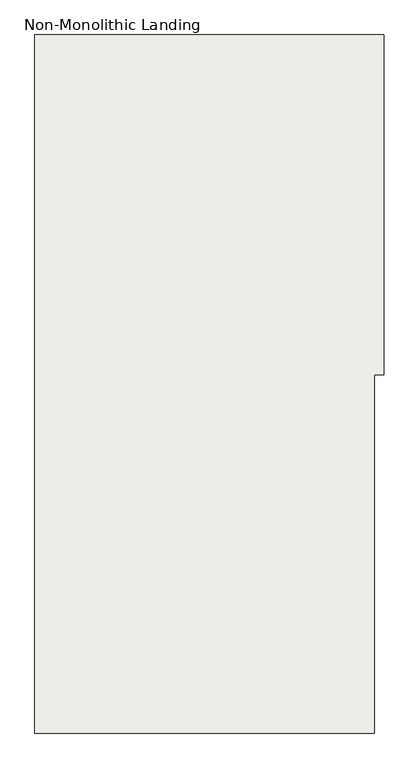
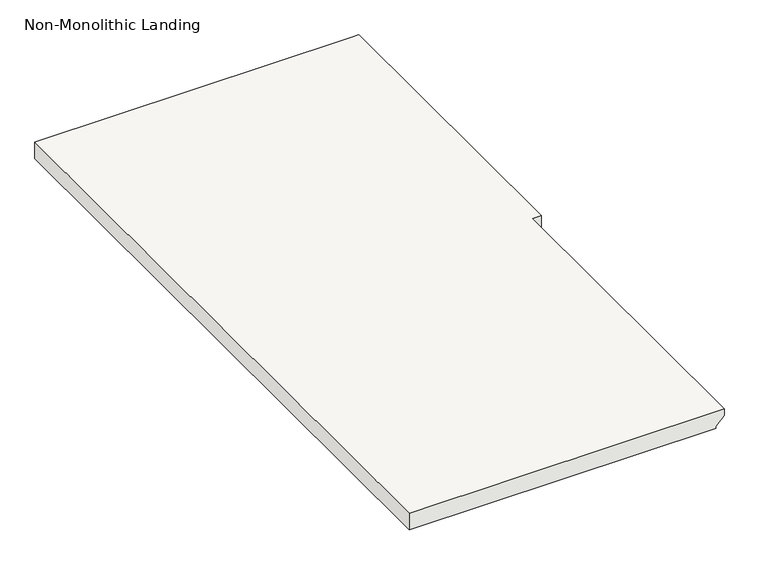
"""IFC4 building model written with IfcOpenShell, lengths in millimetres: slab geometry, Non-Monolithic Landing."""

from ifc_helpers import new_model, si_unit, origin, place, context, project, spatial, faceted_brep, source, transform, mapped, element, save


def non_monolithic_landing_7588ffe4(model_context):
    return source(origin(), model_context, "Body", "Brep", [
        faceted_brep([(-6548.9591614, -562.2450563, 1581.15), (-6574.3591614, -562.2450563, 1555.75), (-6574.3591614, 352.1549437, 1555.75), (-6548.9591614, 352.1549437, 1581.15), (-6548.9591614, 402.4325188, 1600.2), (-6523.5591614, 402.4325188, 1600.2), (-6523.5591614, 1316.8325188, 1600.2), (-6548.9591614, 1316.8325188, 1600.2), (-7463.3591614, 1316.8325188, 1600.2), (-7463.3591614, -562.2450563, 1600.2), (-6548.9591614, -562.2450563, 1600.2), (-6574.3591614, 352.1549437, 1549.4), (-6574.3591614, -562.2450563, 1549.4), (-7463.3591614, -562.2450563, 1549.4), (-7463.3591614, 1316.8325188, 1549.4), (-6548.9591614, 1316.8325188, 1549.4), (-6523.5591614, 1316.8325188, 1549.4), (-6523.5591614, 402.4325188, 1549.4), (-6548.9591614, 402.4325188, 1549.4), (-6548.9591614, 352.1549437, 1549.4)], [[[0, 1, 2, 3]], [[4, 5, 6, 7, 8, 9, 10]], [[11, 12, 13, 14, 15, 16, 17, 18, 19]], [[12, 11, 2, 1]], [[11, 19, 3, 2]], [[4, 10, 0, 3, 19, 18]], [[5, 4, 18, 17]], [[6, 5, 17, 16]], [[7, 6, 16, 15]], [[8, 7, 15, 14]], [[9, 8, 14, 13]], [[10, 9, 13, 12, 1, 0]]]),
    ])


if __name__ == "__main__":
    model = new_model("IFC4")
    model_context = context("Model", 3, world=origin())
    ifc_project = project(units=[si_unit("LENGTHUNIT", "METRE", prefix="MILLI")], contexts=[model_context])
    site = spatial("IfcSite", under=ifc_project)
    building = spatial("IfcBuilding", under=site)
    placement = place(None, origin())
    non_monolithic_landing_shape = non_monolithic_landing_7588ffe4(model_context)
    element("IfcSlab", 1, ObjectType="Non-Monolithic Landing", at=placement, inside=building, context=model_context, shape_type="MappedRepresentation", body=[
        mapped(non_monolithic_landing_shape, transform((0.0, 0.0, 0.0), x_axis=(1.0, 0.0, 0.0), y_axis=(0.0, 1.0, 0.0), z_axis=(0.0, 0.0, 1.0))),
    ])
    save(model, "model.ifc")
